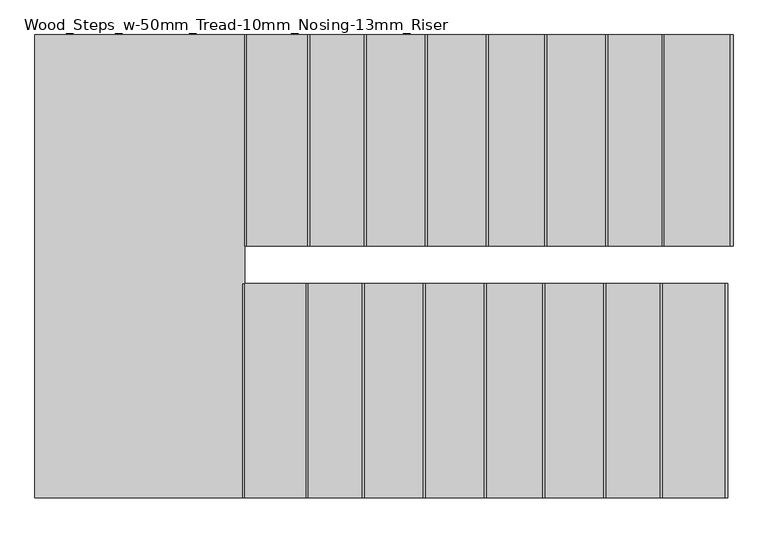
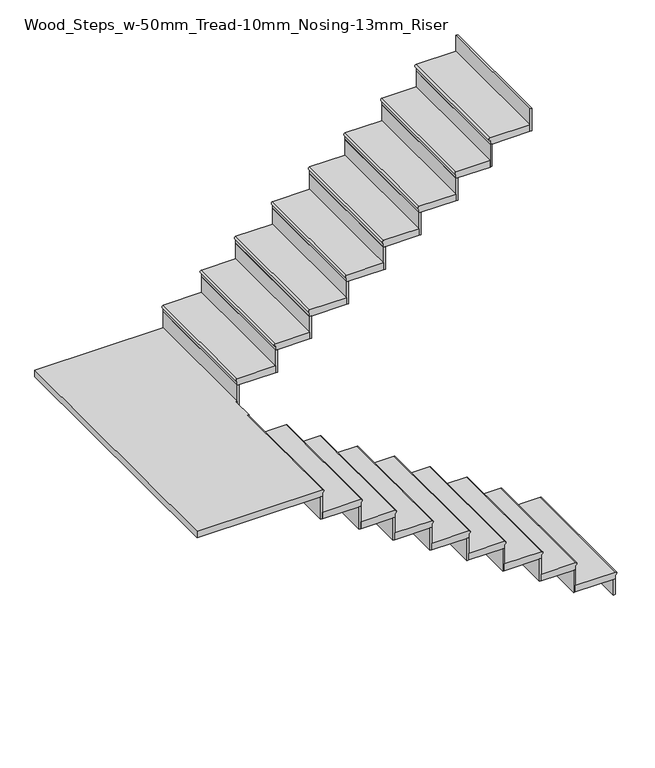
"""IFC4 building model written with IfcOpenShell, lengths in millimetres: stair flight geometry, Wood_Steps_w-50mm_Tread-10mm_Nosing-13mm_Riser."""

from ifc_helpers import new_model, si_unit, frame, origin, place, context, project, spatial, circle_curve, faceted_brep, source, transform, mapped, element, save
from ifc_brep_helpers import plane_surface, cylinder_surface, advanced_brep


def wood_steps_w_50mm_tread_10mm_nosing_13mm_riser_d55d0cb6(model_context):
    return source(origin(), model_context, "Body", "SolidModel", [
        advanced_brep(
        [(-5491.4951322, 1486.5182736, 146.6666667), (-5491.4951322, 1486.5182736, 166.6666667), (-5491.4951322, 572.7642586, 166.6666667), (-5491.4951322, 572.7642586, 146.6666667), (-5771.4951322, 572.7642586, 166.6666667), (-5771.4951322, 1486.5182736, 166.6666667), (-5491.4951322, 572.7642586, 116.6666667), (-5771.4951322, 572.7642586, 116.6666667), (-5771.4951322, 1486.5182736, 116.6666667), (-5491.4951322, 1486.5182736, 116.6666667)],
        [
            (0, 1, circle_curve(frame((-5491.4951322, 1486.5182736, 156.6666667), z_axis=(0.0, -1.0, 0.0), x_axis=(-1.0, 0.0, 0.0)), 10.0)),
            (1, 2),
            (2, 3, circle_curve(frame((-5491.4951322, 572.7642586, 156.6666667), z_axis=(0.0, 1.0, 0.0), x_axis=(-1.0, 0.0, 0.0)), 10.0)),
            (3, 0),
            (4, 2),
            (1, 5),
            (5, 4),
            (6, 7),
            (7, 8),
            (8, 9),
            (9, 6),
            (4, 7),
            (6, 3),
            (9, 0),
            (8, 5),
        ],
        [
            cylinder_surface(frame((-5491.4951322, 1486.5182736, 156.6666667), z_axis=(0.0, 1.0, 0.0), x_axis=(-1.0, 0.0, 0.0)), 10.0),
            plane_surface(frame((-5466.6718965, 572.7642586, 166.6666667), z_axis=(0.0, 0.0, 1.0), x_axis=(1.0, 0.0, 0.0))),
            plane_surface(frame((-5466.6718965, 572.7642586, 116.6666667), z_axis=(0.0, 0.0, -1.0), x_axis=(-1.0, 0.0, 0.0))),
            plane_surface(frame((-5771.4951322, 572.7642586, 166.6666667), z_axis=(0.0, -1.0, 0.0), x_axis=(0.0, 0.0, -1.0))),
            plane_surface(frame((-5491.4951322, 572.7642586, 166.6666667), z_axis=(1.0, 0.0, 0.0), x_axis=(0.0, 0.0, -1.0))),
            plane_surface(frame((-5491.4951322, 1486.5182736, 166.6666667), z_axis=(0.0, 1.0, 0.0), x_axis=(0.0, 0.0, -1.0))),
            plane_surface(frame((-5771.4951322, 1486.5182736, 166.6666667), z_axis=(-1.0, 0.0, 0.0), x_axis=(0.0, 0.0, -1.0))),
        ],
        [
            (0, [[1, 2, 3, 4]]),
            (1, [[5, -2, 6, 7]]),
            (2, [[8, 9, 10, 11]]),
            (3, [[-5, 12, -8, 13, -3]]),
            (4, [[-11, 14, -4, -13]]),
            (5, [[-6, -1, -14, -10, 15]]),
            (6, [[-7, -15, -9, -12]]),
        ],
    ),
        faceted_brep([(-5491.4951322, 1486.5182736, 116.6666667), (-5491.4951322, 1486.5182736, 0.0), (-5503.9951322, 1486.5182736, 0.0), (-5503.9951322, 1486.5182736, 116.6666667), (-5491.4951322, 572.7642586, 116.6666667), (-5503.9951322, 572.7642586, 116.6666667), (-5503.9951322, 572.7642586, 0.0), (-5491.4951322, 572.7642586, 0.0)], [[[0, 1, 2, 3]], [[4, 5, 6, 7]], [[1, 0, 4, 7]], [[2, 1, 7, 6]], [[3, 2, 6, 5]], [[0, 3, 5, 4]]]),
        faceted_brep([(-5771.4951322, 1486.5182736, 283.3333333), (-5771.4951322, 1486.5182736, 116.6666667), (-5783.9951322, 1486.5182736, 116.6666667), (-5783.9951322, 1486.5182736, 283.3333333), (-5771.4951322, 572.7642586, 283.3333333), (-5783.9951322, 572.7642586, 283.3333333), (-5783.9951322, 572.7642586, 116.6666667), (-5771.4951322, 572.7642586, 116.6666667)], [[[0, 1, 2, 3]], [[4, 5, 6, 7]], [[1, 0, 4, 7]], [[2, 1, 7, 6]], [[3, 2, 6, 5]], [[0, 3, 5, 4]]]),
        advanced_brep(
        [(-6011.4951322, 572.7642586, 333.3333333), (-5771.4951322, 572.7642586, 333.3333333), (-5771.4951322, 1486.5182736, 333.3333333), (-6011.4951322, 1486.5182736, 333.3333333), (-5771.4951322, 572.7642586, 283.3333333), (-6011.4951322, 572.7642586, 283.3333333), (-6011.4951322, 1486.5182736, 283.3333333), (-5771.4951322, 1486.5182736, 283.3333333), (-5771.4951322, 572.7642586, 313.3333333), (-5771.4951322, 1486.5182736, 313.3333333)],
        [
            (0, 1),
            (1, 2),
            (2, 3),
            (3, 0),
            (4, 5),
            (5, 6),
            (6, 7),
            (7, 4),
            (0, 5),
            (4, 8),
            (8, 1, circle_curve(frame((-5771.4951322, 572.7642586, 323.3333333), z_axis=(0.0, -1.0, 0.0), x_axis=(-1.0, 0.0, 0.0)), 10.0)),
            (7, 9),
            (9, 8),
            (2, 9, circle_curve(frame((-5771.4951322, 1486.5182736, 323.3333333), z_axis=(0.0, 1.0, 0.0), x_axis=(-1.0, 0.0, 0.0)), 10.0)),
            (6, 3),
        ],
        [
            plane_surface(frame((-5466.6718965, 572.7642586, 333.3333333), z_axis=(0.0, 0.0, 1.0), x_axis=(1.0, 0.0, 0.0))),
            plane_surface(frame((-5466.6718965, 572.7642586, 283.3333333), z_axis=(0.0, 0.0, -1.0), x_axis=(-1.0, 0.0, 0.0))),
            plane_surface(frame((-6011.4951322, 572.7642586, 333.3333333), z_axis=(0.0, -1.0, 0.0), x_axis=(0.0, 0.0, -1.0))),
            plane_surface(frame((-5771.4951322, 572.7642586, 333.3333333), z_axis=(1.0, 0.0, 0.0), x_axis=(0.0, 0.0, -1.0))),
            plane_surface(frame((-5771.4951322, 1486.5182736, 333.3333333), z_axis=(0.0, 1.0, 0.0), x_axis=(0.0, 0.0, -1.0))),
            plane_surface(frame((-6011.4951322, 1486.5182736, 333.3333333), z_axis=(-1.0, 0.0, 0.0), x_axis=(0.0, 0.0, -1.0))),
            cylinder_surface(frame((-5771.4951322, 1486.5182736, 323.3333333), z_axis=(0.0, 1.0, 0.0), x_axis=(-1.0, 0.0, 0.0)), 10.0),
        ],
        [
            (0, [[1, 2, 3, 4]]),
            (1, [[5, 6, 7, 8]]),
            (2, [[-1, 9, -5, 10, 11]]),
            (3, [[-8, 12, 13, -10]]),
            (4, [[-3, 14, -12, -7, 15]]),
            (5, [[-4, -15, -6, -9]]),
            (6, [[-14, -2, -11, -13]]),
        ],
    ),
        faceted_brep([(-6011.4951322, 1486.5182736, 450.0), (-6011.4951322, 1486.5182736, 283.3333333), (-6023.9951322, 1486.5182736, 283.3333333), (-6023.9951322, 1486.5182736, 450.0), (-6011.4951322, 572.7642586, 450.0), (-6023.9951322, 572.7642586, 450.0), (-6023.9951322, 572.7642586, 283.3333333), (-6011.4951322, 572.7642586, 283.3333333)], [[[0, 1, 2, 3]], [[4, 5, 6, 7]], [[1, 0, 4, 7]], [[2, 1, 7, 6]], [[3, 2, 6, 5]], [[0, 3, 5, 4]]]),
        advanced_brep(
        [(-6271.4951322, 572.7642586, 500.0), (-6011.4951322, 572.7642586, 500.0), (-6011.4951322, 1486.5182736, 500.0), (-6271.4951322, 1486.5182736, 500.0), (-6011.4951322, 572.7642586, 450.0), (-6271.4951322, 572.7642586, 450.0), (-6271.4951322, 1486.5182736, 450.0), (-6011.4951322, 1486.5182736, 450.0), (-6011.4951322, 572.7642586, 480.0), (-6011.4951322, 1486.5182736, 480.0)],
        [
            (0, 1),
            (1, 2),
            (2, 3),
            (3, 0),
            (4, 5),
            (5, 6),
            (6, 7),
            (7, 4),
            (0, 5),
            (4, 8),
            (8, 1, circle_curve(frame((-6011.4951322, 572.7642586, 490.0), z_axis=(0.0, -1.0, 0.0), x_axis=(-1.0, 0.0, 0.0)), 10.0)),
            (7, 9),
            (9, 8),
            (2, 9, circle_curve(frame((-6011.4951322, 1486.5182736, 490.0), z_axis=(0.0, 1.0, 0.0), x_axis=(-1.0, 0.0, 0.0)), 10.0)),
            (6, 3),
        ],
        [
            plane_surface(frame((-5466.6718965, 572.7642586, 500.0), z_axis=(0.0, 0.0, 1.0), x_axis=(1.0, 0.0, 0.0))),
            plane_surface(frame((-5466.6718965, 572.7642586, 450.0), z_axis=(0.0, 0.0, -1.0), x_axis=(-1.0, 0.0, 0.0))),
            plane_surface(frame((-6271.4951322, 572.7642586, 500.0), z_axis=(0.0, -1.0, 0.0), x_axis=(0.0, 0.0, -1.0))),
            plane_surface(frame((-6011.4951322, 572.7642586, 500.0), z_axis=(1.0, 0.0, 0.0), x_axis=(0.0, 0.0, -1.0))),
            plane_surface(frame((-6011.4951322, 1486.5182736, 500.0), z_axis=(0.0, 1.0, 0.0), x_axis=(0.0, 0.0, -1.0))),
            plane_surface(frame((-6271.4951322, 1486.5182736, 500.0), z_axis=(-1.0, 0.0, 0.0), x_axis=(0.0, 0.0, -1.0))),
            cylinder_surface(frame((-6011.4951322, 1486.5182736, 490.0), z_axis=(0.0, 1.0, 0.0), x_axis=(-1.0, 0.0, 0.0)), 10.0),
        ],
        [
            (0, [[1, 2, 3, 4]]),
            (1, [[5, 6, 7, 8]]),
            (2, [[-1, 9, -5, 10, 11]]),
            (3, [[-8, 12, 13, -10]]),
            (4, [[-3, 14, -12, -7, 15]]),
            (5, [[-4, -15, -6, -9]]),
            (6, [[-14, -2, -11, -13]]),
        ],
    ),
        faceted_brep([(-6271.4951322, 1486.5182736, 616.6666667), (-6271.4951322, 1486.5182736, 450.0), (-6283.9951322, 1486.5182736, 450.0), (-6283.9951322, 1486.5182736, 616.6666667), (-6271.4951322, 572.7642586, 616.6666667), (-6283.9951322, 572.7642586, 616.6666667), (-6283.9951322, 572.7642586, 450.0), (-6271.4951322, 572.7642586, 450.0)], [[[0, 1, 2, 3]], [[4, 5, 6, 7]], [[1, 0, 4, 7]], [[2, 1, 7, 6]], [[3, 2, 6, 5]], [[0, 3, 5, 4]]]),
        advanced_brep(
        [(-6521.4951322, 572.7642586, 666.6666667), (-6271.4951322, 572.7642586, 666.6666667), (-6271.4951322, 1486.5182736, 666.6666667), (-6521.4951322, 1486.5182736, 666.6666667), (-6271.4951322, 572.7642586, 616.6666667), (-6521.4951322, 572.7642586, 616.6666667), (-6521.4951322, 1486.5182736, 616.6666667), (-6271.4951322, 1486.5182736, 616.6666667), (-6271.4951322, 572.7642586, 646.6666667), (-6271.4951322, 1486.5182736, 646.6666667)],
        [
            (0, 1),
            (1, 2),
            (2, 3),
            (3, 0),
            (4, 5),
            (5, 6),
            (6, 7),
            (7, 4),
            (0, 5),
            (4, 8),
            (8, 1, circle_curve(frame((-6271.4951322, 572.7642586, 656.6666667), z_axis=(0.0, -1.0, 0.0), x_axis=(-1.0, 0.0, 0.0)), 10.0)),
            (7, 9),
            (9, 8),
            (2, 9, circle_curve(frame((-6271.4951322, 1486.5182736, 656.6666667), z_axis=(0.0, 1.0, 0.0), x_axis=(-1.0, 0.0, 0.0)), 10.0)),
            (6, 3),
        ],
        [
            plane_surface(frame((-5466.6718965, 572.7642586, 666.6666667), z_axis=(0.0, 0.0, 1.0), x_axis=(1.0, 0.0, 0.0))),
            plane_surface(frame((-5466.6718965, 572.7642586, 616.6666667), z_axis=(0.0, 0.0, -1.0), x_axis=(-1.0, 0.0, 0.0))),
            plane_surface(frame((-6521.4951322, 572.7642586, 666.6666667), z_axis=(0.0, -1.0, 0.0), x_axis=(0.0, 0.0, -1.0))),
            plane_surface(frame((-6271.4951322, 572.7642586, 666.6666667), z_axis=(1.0, 0.0, 0.0), x_axis=(0.0, 0.0, -1.0))),
            plane_surface(frame((-6271.4951322, 1486.5182736, 666.6666667), z_axis=(0.0, 1.0, 0.0), x_axis=(0.0, 0.0, -1.0))),
            plane_surface(frame((-6521.4951322, 1486.5182736, 666.6666667), z_axis=(-1.0, 0.0, 0.0), x_axis=(0.0, 0.0, -1.0))),
            cylinder_surface(frame((-6271.4951322, 1486.5182736, 656.6666667), z_axis=(0.0, 1.0, 0.0), x_axis=(-1.0, 0.0, 0.0)), 10.0),
        ],
        [
            (0, [[1, 2, 3, 4]]),
            (1, [[5, 6, 7, 8]]),
            (2, [[-1, 9, -5, 10, 11]]),
            (3, [[-8, 12, 13, -10]]),
            (4, [[-3, 14, -12, -7, 15]]),
            (5, [[-4, -15, -6, -9]]),
            (6, [[-14, -2, -11, -13]]),
        ],
    ),
        faceted_brep([(-6521.4951322, 1486.5182736, 783.3333333), (-6521.4951322, 1486.5182736, 616.6666667), (-6533.9951322, 1486.5182736, 616.6666667), (-6533.9951322, 1486.5182736, 783.3333333), (-6521.4951322, 572.7642586, 783.3333333), (-6533.9951322, 572.7642586, 783.3333333), (-6533.9951322, 572.7642586, 616.6666667), (-6521.4951322, 572.7642586, 616.6666667)], [[[0, 1, 2, 3]], [[4, 5, 6, 7]], [[1, 0, 4, 7]], [[2, 1, 7, 6]], [[3, 2, 6, 5]], [[0, 3, 5, 4]]]),
        advanced_brep(
        [(-6781.4951322, 572.7642586, 833.3333333), (-6521.4951322, 572.7642586, 833.3333333), (-6521.4951322, 1486.5182736, 833.3333333), (-6781.4951322, 1486.5182736, 833.3333333), (-6521.4951322, 572.7642586, 783.3333333), (-6781.4951322, 572.7642586, 783.3333333), (-6781.4951322, 1486.5182736, 783.3333333), (-6521.4951322, 1486.5182736, 783.3333333), (-6521.4951322, 572.7642586, 813.3333333), (-6521.4951322, 1486.5182736, 813.3333333)],
        [
            (0, 1),
            (1, 2),
            (2, 3),
            (3, 0),
            (4, 5),
            (5, 6),
            (6, 7),
            (7, 4),
            (0, 5),
            (4, 8),
            (8, 1, circle_curve(frame((-6521.4951322, 572.7642586, 823.3333333), z_axis=(0.0, -1.0, 0.0), x_axis=(-1.0, 0.0, 0.0)), 10.0)),
            (7, 9),
            (9, 8),
            (2, 9, circle_curve(frame((-6521.4951322, 1486.5182736, 823.3333333), z_axis=(0.0, 1.0, 0.0), x_axis=(-1.0, 0.0, 0.0)), 10.0)),
            (6, 3),
        ],
        [
            plane_surface(frame((-5466.6718965, 572.7642586, 833.3333333), z_axis=(0.0, 0.0, 1.0), x_axis=(1.0, 0.0, 0.0))),
            plane_surface(frame((-5466.6718965, 572.7642586, 783.3333333), z_axis=(0.0, 0.0, -1.0), x_axis=(-1.0, 0.0, 0.0))),
            plane_surface(frame((-6781.4951322, 572.7642586, 833.3333333), z_axis=(0.0, -1.0, 0.0), x_axis=(0.0, 0.0, -1.0))),
            plane_surface(frame((-6521.4951322, 572.7642586, 833.3333333), z_axis=(1.0, 0.0, 0.0), x_axis=(0.0, 0.0, -1.0))),
            plane_surface(frame((-6521.4951322, 1486.5182736, 833.3333333), z_axis=(0.0, 1.0, 0.0), x_axis=(0.0, 0.0, -1.0))),
            plane_surface(frame((-6781.4951322, 1486.5182736, 833.3333333), z_axis=(-1.0, 0.0, 0.0), x_axis=(0.0, 0.0, -1.0))),
            cylinder_surface(frame((-6521.4951322, 1486.5182736, 823.3333333), z_axis=(0.0, 1.0, 0.0), x_axis=(-1.0, 0.0, 0.0)), 10.0),
        ],
        [
            (0, [[1, 2, 3, 4]]),
            (1, [[5, 6, 7, 8]]),
            (2, [[-1, 9, -5, 10, 11]]),
            (3, [[-8, 12, 13, -10]]),
            (4, [[-3, 14, -12, -7, 15]]),
            (5, [[-4, -15, -6, -9]]),
            (6, [[-14, -2, -11, -13]]),
        ],
    ),
        faceted_brep([(-6781.4951322, 1486.5182736, 950.0), (-6781.4951322, 1486.5182736, 783.3333333), (-6793.9951322, 1486.5182736, 783.3333333), (-6793.9951322, 1486.5182736, 950.0), (-6781.4951322, 572.7642586, 950.0), (-6793.9951322, 572.7642586, 950.0), (-6793.9951322, 572.7642586, 783.3333333), (-6781.4951322, 572.7642586, 783.3333333)], [[[0, 1, 2, 3]], [[4, 5, 6, 7]], [[1, 0, 4, 7]], [[2, 1, 7, 6]], [[3, 2, 6, 5]], [[0, 3, 5, 4]]]),
        advanced_brep(
        [(-7041.4951322, 572.7642586, 1000.0), (-6781.4951322, 572.7642586, 1000.0), (-6781.4951322, 1486.5182736, 1000.0), (-7041.4951322, 1486.5182736, 1000.0), (-6781.4951322, 572.7642586, 950.0), (-7041.4951322, 572.7642586, 950.0), (-7041.4951322, 1486.5182736, 950.0), (-6781.4951322, 1486.5182736, 950.0), (-6781.4951322, 572.7642586, 980.0), (-6781.4951322, 1486.5182736, 980.0)],
        [
            (0, 1),
            (1, 2),
            (2, 3),
            (3, 0),
            (4, 5),
            (5, 6),
            (6, 7),
            (7, 4),
            (0, 5),
            (4, 8),
            (8, 1, circle_curve(frame((-6781.4951322, 572.7642586, 990.0), z_axis=(0.0, -1.0, 0.0), x_axis=(-1.0, 0.0, 0.0)), 10.0)),
            (7, 9),
            (9, 8),
            (2, 9, circle_curve(frame((-6781.4951322, 1486.5182736, 990.0), z_axis=(0.0, 1.0, 0.0), x_axis=(-1.0, 0.0, 0.0)), 10.0)),
            (6, 3),
        ],
        [
            plane_surface(frame((-5726.6718965, 572.7642586, 1000.0), z_axis=(0.0, 0.0, 1.0), x_axis=(1.0, 0.0, 0.0))),
            plane_surface(frame((-5726.6718965, 572.7642586, 950.0), z_axis=(0.0, 0.0, -1.0), x_axis=(-1.0, 0.0, 0.0))),
            plane_surface(frame((-7041.4951322, 572.7642586, 1000.0), z_axis=(0.0, -1.0, 0.0), x_axis=(0.0, 0.0, -1.0))),
            plane_surface(frame((-6781.4951322, 572.7642586, 1000.0), z_axis=(1.0, 0.0, 0.0), x_axis=(0.0, 0.0, -1.0))),
            plane_surface(frame((-6781.4951322, 1486.5182736, 1000.0), z_axis=(0.0, 1.0, 0.0), x_axis=(0.0, 0.0, -1.0))),
            plane_surface(frame((-7041.4951322, 1486.5182736, 1000.0), z_axis=(-1.0, 0.0, 0.0), x_axis=(0.0, 0.0, -1.0))),
            cylinder_surface(frame((-6781.4951322, 1486.5182736, 990.0), z_axis=(0.0, 1.0, 0.0), x_axis=(-1.0, 0.0, 0.0)), 10.0),
        ],
        [
            (0, [[1, 2, 3, 4]]),
            (1, [[5, 6, 7, 8]]),
            (2, [[-1, 9, -5, 10, 11]]),
            (3, [[-8, 12, 13, -10]]),
            (4, [[-3, 14, -12, -7, 15]]),
            (5, [[-4, -15, -6, -9]]),
            (6, [[-14, -2, -11, -13]]),
        ],
    ),
        faceted_brep([(-7041.4951322, 1486.5182736, 1116.6666667), (-7041.4951322, 1486.5182736, 950.0), (-7053.9951322, 1486.5182736, 950.0), (-7053.9951322, 1486.5182736, 1116.6666667), (-7041.4951322, 572.7642586, 1116.6666667), (-7053.9951322, 572.7642586, 1116.6666667), (-7053.9951322, 572.7642586, 950.0), (-7041.4951322, 572.7642586, 950.0)], [[[0, 1, 2, 3]], [[4, 5, 6, 7]], [[1, 0, 4, 7]], [[2, 1, 7, 6]], [[3, 2, 6, 5]], [[0, 3, 5, 4]]]),
        advanced_brep(
        [(-7281.4951322, 572.7642586, 1166.6666667), (-7041.4951322, 572.7642586, 1166.6666667), (-7041.4951322, 1486.5182736, 1166.6666667), (-7281.4951322, 1486.5182736, 1166.6666667), (-7041.4951322, 572.7642586, 1116.6666667), (-7281.4951322, 572.7642586, 1116.6666667), (-7281.4951322, 1486.5182736, 1116.6666667), (-7041.4951322, 1486.5182736, 1116.6666667), (-7041.4951322, 572.7642586, 1146.6666667), (-7041.4951322, 1486.5182736, 1146.6666667)],
        [
            (0, 1),
            (1, 2),
            (2, 3),
            (3, 0),
            (4, 5),
            (5, 6),
            (6, 7),
            (7, 4),
            (0, 5),
            (4, 8),
            (8, 1, circle_curve(frame((-7041.4951322, 572.7642586, 1156.6666667), z_axis=(0.0, -1.0, 0.0), x_axis=(-1.0, 0.0, 0.0)), 10.0)),
            (7, 9),
            (9, 8),
            (2, 9, circle_curve(frame((-7041.4951322, 1486.5182736, 1156.6666667), z_axis=(0.0, 1.0, 0.0), x_axis=(-1.0, 0.0, 0.0)), 10.0)),
            (6, 3),
        ],
        [
            plane_surface(frame((-5466.6718965, 572.7642586, 1166.6666667), z_axis=(0.0, 0.0, 1.0), x_axis=(1.0, 0.0, 0.0))),
            plane_surface(frame((-5466.6718965, 572.7642586, 1116.6666667), z_axis=(0.0, 0.0, -1.0), x_axis=(-1.0, 0.0, 0.0))),
            plane_surface(frame((-7281.4951322, 572.7642586, 1166.6666667), z_axis=(0.0, -1.0, 0.0), x_axis=(0.0, 0.0, -1.0))),
            plane_surface(frame((-7041.4951322, 572.7642586, 1166.6666667), z_axis=(1.0, 0.0, 0.0), x_axis=(0.0, 0.0, -1.0))),
            plane_surface(frame((-7041.4951322, 1486.5182736, 1166.6666667), z_axis=(0.0, 1.0, 0.0), x_axis=(0.0, 0.0, -1.0))),
            plane_surface(frame((-7281.4951322, 1486.5182736, 1166.6666667), z_axis=(-1.0, 0.0, 0.0), x_axis=(0.0, 0.0, -1.0))),
            cylinder_surface(frame((-7041.4951322, 1486.5182736, 1156.6666667), z_axis=(0.0, 1.0, 0.0), x_axis=(-1.0, 0.0, 0.0)), 10.0),
        ],
        [
            (0, [[1, 2, 3, 4]]),
            (1, [[5, 6, 7, 8]]),
            (2, [[-1, 9, -5, 10, 11]]),
            (3, [[-8, 12, 13, -10]]),
            (4, [[-3, 14, -12, -7, 15]]),
            (5, [[-4, -15, -6, -9]]),
            (6, [[-14, -2, -11, -13]]),
        ],
    ),
        faceted_brep([(-7281.4951322, 1486.5182736, 1283.3333333), (-7281.4951322, 1486.5182736, 1116.6666667), (-7293.9951322, 1486.5182736, 1116.6666667), (-7293.9951322, 1486.5182736, 1283.3333333), (-7281.4951322, 572.7642586, 1283.3333333), (-7293.9951322, 572.7642586, 1283.3333333), (-7293.9951322, 572.7642586, 1116.6666667), (-7281.4951322, 572.7642586, 1116.6666667)], [[[0, 1, 2, 3]], [[4, 5, 6, 7]], [[1, 0, 4, 7]], [[2, 1, 7, 6]], [[3, 2, 6, 5]], [[0, 3, 5, 4]]]),
        advanced_brep(
        [(-7551.4951322, 572.7642586, 1333.3333333), (-7281.4951322, 572.7642586, 1333.3333333), (-7281.4951322, 1486.5182736, 1333.3333333), (-7551.4951322, 1486.5182736, 1333.3333333), (-7281.4951322, 572.7642586, 1283.3333333), (-7551.4951322, 572.7642586, 1283.3333333), (-7551.4951322, 1486.5182736, 1283.3333333), (-7281.4951322, 1486.5182736, 1283.3333333), (-7281.4951322, 572.7642586, 1313.3333333), (-7281.4951322, 1486.5182736, 1313.3333333)],
        [
            (0, 1),
            (1, 2),
            (2, 3),
            (3, 0),
            (4, 5),
            (5, 6),
            (6, 7),
            (7, 4),
            (0, 5),
            (4, 8),
            (8, 1, circle_curve(frame((-7281.4951322, 572.7642586, 1323.3333333), z_axis=(0.0, -1.0, 0.0), x_axis=(-1.0, 0.0, 0.0)), 10.0)),
            (7, 9),
            (9, 8),
            (2, 9, circle_curve(frame((-7281.4951322, 1486.5182736, 1323.3333333), z_axis=(0.0, 1.0, 0.0), x_axis=(-1.0, 0.0, 0.0)), 10.0)),
            (6, 3),
        ],
        [
            plane_surface(frame((-5466.6718965, 572.7642586, 1333.3333333), z_axis=(0.0, 0.0, 1.0), x_axis=(1.0, 0.0, 0.0))),
            plane_surface(frame((-5466.6718965, 572.7642586, 1283.3333333), z_axis=(0.0, 0.0, -1.0), x_axis=(-1.0, 0.0, 0.0))),
            plane_surface(frame((-7551.4951322, 572.7642586, 1333.3333333), z_axis=(0.0, -1.0, 0.0), x_axis=(0.0, 0.0, -1.0))),
            plane_surface(frame((-7281.4951322, 572.7642586, 1333.3333333), z_axis=(1.0, 0.0, 0.0), x_axis=(0.0, 0.0, -1.0))),
            plane_surface(frame((-7281.4951322, 1486.5182736, 1333.3333333), z_axis=(0.0, 1.0, 0.0), x_axis=(0.0, 0.0, -1.0))),
            plane_surface(frame((-7551.4951322, 1486.5182736, 1333.3333333), z_axis=(-1.0, 0.0, 0.0), x_axis=(0.0, 0.0, -1.0))),
            cylinder_surface(frame((-7281.4951322, 1486.5182736, 1323.3333333), z_axis=(0.0, 1.0, 0.0), x_axis=(-1.0, 0.0, 0.0)), 10.0),
        ],
        [
            (0, [[1, 2, 3, 4]]),
            (1, [[5, 6, 7, 8]]),
            (2, [[-1, 9, -5, 10, 11]]),
            (3, [[-8, 12, 13, -10]]),
            (4, [[-3, 14, -12, -7, 15]]),
            (5, [[-4, -15, -6, -9]]),
            (6, [[-14, -2, -11, -13]]),
        ],
    ),
        faceted_brep([(-7551.4951322, 1486.5182736, 1450.0), (-7551.4951322, 1486.5182736, 1283.3333333), (-7563.9951322, 1486.5182736, 1283.3333333), (-7563.9951322, 1486.5182736, 1450.0), (-7551.4951322, 572.7642586, 1450.0), (-7563.9951322, 572.7642586, 1450.0), (-7563.9951322, 572.7642586, 1283.3333333), (-7551.4951322, 572.7642586, 1283.3333333)], [[[0, 1, 2, 3]], [[4, 5, 6, 7]], [[1, 0, 4, 7]], [[2, 1, 7, 6]], [[3, 2, 6, 5]], [[0, 3, 5, 4]]]),
        advanced_brep(
        [(-7531.4951322, 2546.998858, 1500.0), (-8434.8904087, 2546.998858, 1500.0), (-8434.8904087, 572.7642586, 1500.0), (-7551.4951322, 572.7642586, 1500.0), (-7551.4951322, 1486.5182736, 1500.0), (-7541.4951322, 1486.5182736, 1500.0), (-7541.4951322, 1646.5182736, 1500.0), (-7531.4951322, 1646.5182736, 1500.0), (-8434.8904087, 2546.998858, 1450.0), (-7531.4951322, 2546.998858, 1450.0), (-7531.4951322, 1646.5182736, 1450.0), (-7541.4951322, 1646.5182736, 1450.0), (-7541.4951322, 1486.5182736, 1450.0), (-7551.4951322, 1486.5182736, 1450.0), (-7551.4951322, 572.7642586, 1450.0), (-8434.8904087, 572.7642586, 1450.0), (-7551.4951322, 572.7642586, 1480.0), (-7551.4951322, 1486.5182736, 1480.0), (-7541.4951322, 1486.5182736, 1490.0)],
        [
            (0, 1),
            (1, 2),
            (2, 3),
            (3, 4),
            (4, 5),
            (5, 6),
            (6, 7),
            (7, 0),
            (8, 9),
            (9, 10),
            (10, 11),
            (11, 12),
            (12, 13),
            (13, 14),
            (14, 15),
            (15, 8),
            (0, 9),
            (8, 1),
            (15, 2),
            (14, 16),
            (16, 3, circle_curve(frame((-7551.4951322, 572.7642586, 1490.0), z_axis=(0.0, -1.0, 0.0), x_axis=(-1.0, 0.0, 0.0)), 10.0)),
            (13, 17),
            (17, 16),
            (4, 18, circle_curve(frame((-7551.4951322, 1486.5182736, 1490.0), z_axis=(0.0, 1.0, 0.0), x_axis=(-1.0, 0.0, 0.0)), 10.0)),
            (18, 5),
            (12, 18),
            (18, 17, circle_curve(frame((-7551.4951322, 1486.5182736, 1490.0), z_axis=(0.0, 1.0, 0.0), x_axis=(-1.0, 0.0, 0.0)), 10.0)),
            (11, 6),
            (10, 7),
        ],
        [
            plane_surface(frame((-8434.8904087, 2546.998858, 1500.0), z_axis=(0.0, 0.0, 1.0), x_axis=(-1.0, 0.0, 0.0))),
            plane_surface(frame((-8434.8904087, 2546.998858, 1450.0), z_axis=(0.0, 0.0, -1.0), x_axis=(1.0, 0.0, 0.0))),
            plane_surface(frame((-7531.4951322, 2546.998858, 1500.0), z_axis=(0.0, 1.0, 0.0), x_axis=(0.0, 0.0, -1.0))),
            plane_surface(frame((-8434.8904087, 2546.998858, 1500.0), z_axis=(-1.0, 0.0, 0.0), x_axis=(0.0, 0.0, -1.0))),
            plane_surface(frame((-8434.8904087, 572.7642586, 1500.0), z_axis=(0.0, -1.0, 0.0), x_axis=(0.0, 0.0, -1.0))),
            plane_surface(frame((-7551.4951322, 572.7642586, 1500.0), z_axis=(1.0, 0.0, 0.0), x_axis=(0.0, 0.0, -1.0))),
            plane_surface(frame((-7551.4951322, 1486.5182736, 1500.0), z_axis=(0.0, -1.0, 0.0), x_axis=(0.0, 0.0, -1.0))),
            plane_surface(frame((-7541.4951322, 1486.5182736, 1500.0), z_axis=(1.0, 0.0, 0.0), x_axis=(0.0, 0.0, -1.0))),
            plane_surface(frame((-7541.4951322, 1646.5182736, 1500.0), z_axis=(0.0, -1.0, 0.0), x_axis=(0.0, 0.0, -1.0))),
            plane_surface(frame((-7531.4951322, 1646.5182736, 1500.0), z_axis=(1.0, 0.0, 0.0), x_axis=(0.0, 0.0, -1.0))),
            cylinder_surface(frame((-7551.4951322, 1486.5182736, 1490.0), z_axis=(0.0, 1.0, 0.0), x_axis=(-1.0, 0.0, 0.0)), 10.0),
        ],
        [
            (0, [[1, 2, 3, 4, 5, 6, 7, 8]]),
            (1, [[9, 10, 11, 12, 13, 14, 15, 16]]),
            (2, [[-1, 17, -9, 18]]),
            (3, [[-2, -18, -16, 19]]),
            (4, [[-3, -19, -15, 20, 21]]),
            (5, [[-14, 22, 23, -20]]),
            (6, [[-5, 24, 25]]),
            (6, [[-13, 26, 27, -22]]),
            (7, [[-6, -25, -26, -12, 28]]),
            (8, [[-7, -28, -11, 29]]),
            (9, [[-8, -29, -10, -17]]),
            (10, [[-21, -23, -27, -24, -4]]),
        ],
    ),
        faceted_brep([(-7531.4951322, 1646.5182736, 1616.6666667), (-7531.4951322, 1646.5182736, 1450.0), (-7518.9951322, 1646.5182736, 1450.0), (-7518.9951322, 1646.5182736, 1616.6666667), (-7531.4951322, 2546.998858, 1616.6666667), (-7518.9951322, 2546.998858, 1616.6666667), (-7518.9951322, 2546.998858, 1450.0), (-7531.4951322, 2546.998858, 1450.0)], [[[0, 1, 2, 3]], [[4, 5, 6, 7]], [[1, 0, 4, 7]], [[2, 1, 7, 6]], [[3, 2, 6, 5]], [[0, 3, 5, 4]]]),
        advanced_brep(
        [(-7261.4951322, 2546.998858, 1666.6666667), (-7531.4951322, 2546.998858, 1666.6666667), (-7531.4951322, 1646.5182736, 1666.6666667), (-7261.4951322, 1646.5182736, 1666.6666667), (-7531.4951322, 2546.998858, 1616.6666667), (-7261.4951322, 2546.998858, 1616.6666667), (-7261.4951322, 1646.5182736, 1616.6666667), (-7531.4951322, 1646.5182736, 1616.6666667), (-7531.4951322, 2546.998858, 1646.6666667), (-7531.4951322, 1646.5182736, 1646.6666667)],
        [
            (0, 1),
            (1, 2),
            (2, 3),
            (3, 0),
            (4, 5),
            (5, 6),
            (6, 7),
            (7, 4),
            (0, 5),
            (4, 8),
            (8, 1, circle_curve(frame((-7531.4951322, 2546.998858, 1656.6666667), z_axis=(0.0, 1.0, 0.0), x_axis=(1.0, 0.0, 0.0)), 10.0)),
            (7, 9),
            (9, 8),
            (2, 9, circle_curve(frame((-7531.4951322, 1646.5182736, 1656.6666667), z_axis=(0.0, -1.0, 0.0), x_axis=(1.0, 0.0, 0.0)), 10.0)),
            (6, 3),
        ],
        [
            plane_surface(frame((-8434.8904087, 2546.998858, 1666.6666667), z_axis=(0.0, 0.0, 1.0), x_axis=(-1.0, 0.0, 0.0))),
            plane_surface(frame((-8434.8904087, 2546.998858, 1616.6666667), z_axis=(0.0, 0.0, -1.0), x_axis=(1.0, 0.0, 0.0))),
            plane_surface(frame((-7261.4951322, 2546.998858, 1666.6666667), z_axis=(0.0, 1.0, 0.0), x_axis=(0.0, 0.0, -1.0))),
            plane_surface(frame((-7531.4951322, 2546.998858, 1666.6666667), z_axis=(-1.0, 0.0, 0.0), x_axis=(0.0, 0.0, -1.0))),
            plane_surface(frame((-7531.4951322, 1646.5182736, 1666.6666667), z_axis=(0.0, -1.0, 0.0), x_axis=(0.0, 0.0, -1.0))),
            plane_surface(frame((-7261.4951322, 1646.5182736, 1666.6666667), z_axis=(1.0, 0.0, 0.0), x_axis=(0.0, 0.0, -1.0))),
            cylinder_surface(frame((-7531.4951322, 1646.5182736, 1656.6666667), z_axis=(0.0, -1.0, 0.0), x_axis=(1.0, 0.0, 0.0)), 10.0),
        ],
        [
            (0, [[1, 2, 3, 4]]),
            (1, [[5, 6, 7, 8]]),
            (2, [[-1, 9, -5, 10, 11]]),
            (3, [[-8, 12, 13, -10]]),
            (4, [[-3, 14, -12, -7, 15]]),
            (5, [[-4, -15, -6, -9]]),
            (6, [[-14, -2, -11, -13]]),
        ],
    ),
        faceted_brep([(-7261.4951322, 1646.5182736, 1783.3333333), (-7261.4951322, 1646.5182736, 1616.6666667), (-7248.9951322, 1646.5182736, 1616.6666667), (-7248.9951322, 1646.5182736, 1783.3333333), (-7261.4951322, 2546.998858, 1783.3333333), (-7248.9951322, 2546.998858, 1783.3333333), (-7248.9951322, 2546.998858, 1616.6666667), (-7261.4951322, 2546.998858, 1616.6666667)], [[[0, 1, 2, 3]], [[4, 5, 6, 7]], [[1, 0, 4, 7]], [[2, 1, 7, 6]], [[3, 2, 6, 5]], [[0, 3, 5, 4]]]),
        advanced_brep(
        [(-7021.4951322, 2546.998858, 1833.3333333), (-7261.4951322, 2546.998858, 1833.3333333), (-7261.4951322, 1646.5182736, 1833.3333333), (-7021.4951322, 1646.5182736, 1833.3333333), (-7261.4951322, 2546.998858, 1783.3333333), (-7021.4951322, 2546.998858, 1783.3333333), (-7021.4951322, 1646.5182736, 1783.3333333), (-7261.4951322, 1646.5182736, 1783.3333333), (-7261.4951322, 2546.998858, 1813.3333333), (-7261.4951322, 1646.5182736, 1813.3333333)],
        [
            (0, 1),
            (1, 2),
            (2, 3),
            (3, 0),
            (4, 5),
            (5, 6),
            (6, 7),
            (7, 4),
            (0, 5),
            (4, 8),
            (8, 1, circle_curve(frame((-7261.4951322, 2546.998858, 1823.3333333), z_axis=(0.0, 1.0, 0.0), x_axis=(1.0, 0.0, 0.0)), 10.0)),
            (7, 9),
            (9, 8),
            (2, 9, circle_curve(frame((-7261.4951322, 1646.5182736, 1823.3333333), z_axis=(0.0, -1.0, 0.0), x_axis=(1.0, 0.0, 0.0)), 10.0)),
            (6, 3),
        ],
        [
            plane_surface(frame((-8434.8904087, 2546.998858, 1833.3333333), z_axis=(0.0, 0.0, 1.0), x_axis=(-1.0, 0.0, 0.0))),
            plane_surface(frame((-8434.8904087, 2546.998858, 1783.3333333), z_axis=(0.0, 0.0, -1.0), x_axis=(1.0, 0.0, 0.0))),
            plane_surface(frame((-7021.4951322, 2546.998858, 1833.3333333), z_axis=(0.0, 1.0, 0.0), x_axis=(0.0, 0.0, -1.0))),
            plane_surface(frame((-7261.4951322, 2546.998858, 1833.3333333), z_axis=(-1.0, 0.0, 0.0), x_axis=(0.0, 0.0, -1.0))),
            plane_surface(frame((-7261.4951322, 1646.5182736, 1833.3333333), z_axis=(0.0, -1.0, 0.0), x_axis=(0.0, 0.0, -1.0))),
            plane_surface(frame((-7021.4951322, 1646.5182736, 1833.3333333), z_axis=(1.0, 0.0, 0.0), x_axis=(0.0, 0.0, -1.0))),
            cylinder_surface(frame((-7261.4951322, 1646.5182736, 1823.3333333), z_axis=(0.0, -1.0, 0.0), x_axis=(1.0, 0.0, 0.0)), 10.0),
        ],
        [
            (0, [[1, 2, 3, 4]]),
            (1, [[5, 6, 7, 8]]),
            (2, [[-1, 9, -5, 10, 11]]),
            (3, [[-8, 12, 13, -10]]),
            (4, [[-3, 14, -12, -7, 15]]),
            (5, [[-4, -15, -6, -9]]),
            (6, [[-14, -2, -11, -13]]),
        ],
    ),
        faceted_brep([(-7021.4951322, 1646.5182736, 1950.0), (-7021.4951322, 1646.5182736, 1783.3333333), (-7008.9951322, 1646.5182736, 1783.3333333), (-7008.9951322, 1646.5182736, 1950.0), (-7021.4951322, 2546.998858, 1950.0), (-7008.9951322, 2546.998858, 1950.0), (-7008.9951322, 2546.998858, 1783.3333333), (-7021.4951322, 2546.998858, 1783.3333333)], [[[0, 1, 2, 3]], [[4, 5, 6, 7]], [[1, 0, 4, 7]], [[2, 1, 7, 6]], [[3, 2, 6, 5]], [[0, 3, 5, 4]]]),
        advanced_brep(
        [(-6761.4951322, 2546.998858, 2000.0), (-7021.4951322, 2546.998858, 2000.0), (-7021.4951322, 1646.5182736, 2000.0), (-6761.4951322, 1646.5182736, 2000.0), (-7021.4951322, 2546.998858, 1950.0), (-6761.4951322, 2546.998858, 1950.0), (-6761.4951322, 1646.5182736, 1950.0), (-7021.4951322, 1646.5182736, 1950.0), (-7021.4951322, 2546.998858, 1980.0), (-7021.4951322, 1646.5182736, 1980.0)],
        [
            (0, 1),
            (1, 2),
            (2, 3),
            (3, 0),
            (4, 5),
            (5, 6),
            (6, 7),
            (7, 4),
            (0, 5),
            (4, 8),
            (8, 1, circle_curve(frame((-7021.4951322, 2546.998858, 1990.0), z_axis=(0.0, 1.0, 0.0), x_axis=(1.0, 0.0, 0.0)), 10.0)),
            (7, 9),
            (9, 8),
            (2, 9, circle_curve(frame((-7021.4951322, 1646.5182736, 1990.0), z_axis=(0.0, -1.0, 0.0), x_axis=(1.0, 0.0, 0.0)), 10.0)),
            (6, 3),
        ],
        [
            plane_surface(frame((-8434.8904087, 2546.998858, 2000.0), z_axis=(0.0, 0.0, 1.0), x_axis=(-1.0, 0.0, 0.0))),
            plane_surface(frame((-8434.8904087, 2546.998858, 1950.0), z_axis=(0.0, 0.0, -1.0), x_axis=(1.0, 0.0, 0.0))),
            plane_surface(frame((-6761.4951322, 2546.998858, 2000.0), z_axis=(0.0, 1.0, 0.0), x_axis=(0.0, 0.0, -1.0))),
            plane_surface(frame((-7021.4951322, 2546.998858, 2000.0), z_axis=(-1.0, 0.0, 0.0), x_axis=(0.0, 0.0, -1.0))),
            plane_surface(frame((-7021.4951322, 1646.5182736, 2000.0), z_axis=(0.0, -1.0, 0.0), x_axis=(0.0, 0.0, -1.0))),
            plane_surface(frame((-6761.4951322, 1646.5182736, 2000.0), z_axis=(1.0, 0.0, 0.0), x_axis=(0.0, 0.0, -1.0))),
            cylinder_surface(frame((-7021.4951322, 1646.5182736, 1990.0), z_axis=(0.0, -1.0, 0.0), x_axis=(1.0, 0.0, 0.0)), 10.0),
        ],
        [
            (0, [[1, 2, 3, 4]]),
            (1, [[5, 6, 7, 8]]),
            (2, [[-1, 9, -5, 10, 11]]),
            (3, [[-8, 12, 13, -10]]),
            (4, [[-3, 14, -12, -7, 15]]),
            (5, [[-4, -15, -6, -9]]),
            (6, [[-14, -2, -11, -13]]),
        ],
    ),
        faceted_brep([(-6761.4951322, 1646.5182736, 2116.6666667), (-6761.4951322, 1646.5182736, 1950.0), (-6748.9951322, 1646.5182736, 1950.0), (-6748.9951322, 1646.5182736, 2116.6666667), (-6761.4951322, 2546.998858, 2116.6666667), (-6748.9951322, 2546.998858, 2116.6666667), (-6748.9951322, 2546.998858, 1950.0), (-6761.4951322, 2546.998858, 1950.0)], [[[0, 1, 2, 3]], [[4, 5, 6, 7]], [[1, 0, 4, 7]], [[2, 1, 7, 6]], [[3, 2, 6, 5]], [[0, 3, 5, 4]]]),
        advanced_brep(
        [(-6501.4951322, 2546.998858, 2166.6666667), (-6761.4951322, 2546.998858, 2166.6666667), (-6761.4951322, 1646.5182736, 2166.6666667), (-6501.4951322, 1646.5182736, 2166.6666667), (-6761.4951322, 2546.998858, 2116.6666667), (-6501.4951322, 2546.998858, 2116.6666667), (-6501.4951322, 1646.5182736, 2116.6666667), (-6761.4951322, 1646.5182736, 2116.6666667), (-6761.4951322, 2546.998858, 2146.6666667), (-6761.4951322, 1646.5182736, 2146.6666667)],
        [
            (0, 1),
            (1, 2),
            (2, 3),
            (3, 0),
            (4, 5),
            (5, 6),
            (6, 7),
            (7, 4),
            (0, 5),
            (4, 8),
            (8, 1, circle_curve(frame((-6761.4951322, 2546.998858, 2156.6666667), z_axis=(0.0, 1.0, 0.0), x_axis=(1.0, 0.0, 0.0)), 10.0)),
            (7, 9),
            (9, 8),
            (2, 9, circle_curve(frame((-6761.4951322, 1646.5182736, 2156.6666667), z_axis=(0.0, -1.0, 0.0), x_axis=(1.0, 0.0, 0.0)), 10.0)),
            (6, 3),
        ],
        [
            plane_surface(frame((-8174.8904087, 2546.998858, 2166.6666667), z_axis=(0.0, 0.0, 1.0), x_axis=(-1.0, 0.0, 0.0))),
            plane_surface(frame((-8174.8904087, 2546.998858, 2116.6666667), z_axis=(0.0, 0.0, -1.0), x_axis=(1.0, 0.0, 0.0))),
            plane_surface(frame((-6501.4951322, 2546.998858, 2166.6666667), z_axis=(0.0, 1.0, 0.0), x_axis=(0.0, 0.0, -1.0))),
            plane_surface(frame((-6761.4951322, 2546.998858, 2166.6666667), z_axis=(-1.0, 0.0, 0.0), x_axis=(0.0, 0.0, -1.0))),
            plane_surface(frame((-6761.4951322, 1646.5182736, 2166.6666667), z_axis=(0.0, -1.0, 0.0), x_axis=(0.0, 0.0, -1.0))),
            plane_surface(frame((-6501.4951322, 1646.5182736, 2166.6666667), z_axis=(1.0, 0.0, 0.0), x_axis=(0.0, 0.0, -1.0))),
            cylinder_surface(frame((-6761.4951322, 1646.5182736, 2156.6666667), z_axis=(0.0, -1.0, 0.0), x_axis=(1.0, 0.0, 0.0)), 10.0),
        ],
        [
            (0, [[1, 2, 3, 4]]),
            (1, [[5, 6, 7, 8]]),
            (2, [[-1, 9, -5, 10, 11]]),
            (3, [[-8, 12, 13, -10]]),
            (4, [[-3, 14, -12, -7, 15]]),
            (5, [[-4, -15, -6, -9]]),
            (6, [[-14, -2, -11, -13]]),
        ],
    ),
        faceted_brep([(-6501.4951322, 1646.5182736, 2283.3333333), (-6501.4951322, 1646.5182736, 2116.6666667), (-6488.9951322, 1646.5182736, 2116.6666667), (-6488.9951322, 1646.5182736, 2283.3333333), (-6501.4951322, 2546.998858, 2283.3333333), (-6488.9951322, 2546.998858, 2283.3333333), (-6488.9951322, 2546.998858, 2116.6666667), (-6501.4951322, 2546.998858, 2116.6666667)], [[[0, 1, 2, 3]], [[4, 5, 6, 7]], [[1, 0, 4, 7]], [[2, 1, 7, 6]], [[3, 2, 6, 5]], [[0, 3, 5, 4]]]),
        advanced_brep(
        [(-6251.4951322, 2546.998858, 2333.3333333), (-6501.4951322, 2546.998858, 2333.3333333), (-6501.4951322, 1646.5182736, 2333.3333333), (-6251.4951322, 1646.5182736, 2333.3333333), (-6501.4951322, 2546.998858, 2283.3333333), (-6251.4951322, 2546.998858, 2283.3333333), (-6251.4951322, 1646.5182736, 2283.3333333), (-6501.4951322, 1646.5182736, 2283.3333333), (-6501.4951322, 2546.998858, 2313.3333333), (-6501.4951322, 1646.5182736, 2313.3333333)],
        [
            (0, 1),
            (1, 2),
            (2, 3),
            (3, 0),
            (4, 5),
            (5, 6),
            (6, 7),
            (7, 4),
            (0, 5),
            (4, 8),
            (8, 1, circle_curve(frame((-6501.4951322, 2546.998858, 2323.3333333), z_axis=(0.0, 1.0, 0.0), x_axis=(1.0, 0.0, 0.0)), 10.0)),
            (7, 9),
            (9, 8),
            (2, 9, circle_curve(frame((-6501.4951322, 1646.5182736, 2323.3333333), z_axis=(0.0, -1.0, 0.0), x_axis=(1.0, 0.0, 0.0)), 10.0)),
            (6, 3),
        ],
        [
            plane_surface(frame((-8434.8904087, 2546.998858, 2333.3333333), z_axis=(0.0, 0.0, 1.0), x_axis=(-1.0, 0.0, 0.0))),
            plane_surface(frame((-8434.8904087, 2546.998858, 2283.3333333), z_axis=(0.0, 0.0, -1.0), x_axis=(1.0, 0.0, 0.0))),
            plane_surface(frame((-6251.4951322, 2546.998858, 2333.3333333), z_axis=(0.0, 1.0, 0.0), x_axis=(0.0, 0.0, -1.0))),
            plane_surface(frame((-6501.4951322, 2546.998858, 2333.3333333), z_axis=(-1.0, 0.0, 0.0), x_axis=(0.0, 0.0, -1.0))),
            plane_surface(frame((-6501.4951322, 1646.5182736, 2333.3333333), z_axis=(0.0, -1.0, 0.0), x_axis=(0.0, 0.0, -1.0))),
            plane_surface(frame((-6251.4951322, 1646.5182736, 2333.3333333), z_axis=(1.0, 0.0, 0.0), x_axis=(0.0, 0.0, -1.0))),
            cylinder_surface(frame((-6501.4951322, 1646.5182736, 2323.3333333), z_axis=(0.0, -1.0, 0.0), x_axis=(1.0, 0.0, 0.0)), 10.0),
        ],
        [
            (0, [[1, 2, 3, 4]]),
            (1, [[5, 6, 7, 8]]),
            (2, [[-1, 9, -5, 10, 11]]),
            (3, [[-8, 12, 13, -10]]),
            (4, [[-3, 14, -12, -7, 15]]),
            (5, [[-4, -15, -6, -9]]),
            (6, [[-14, -2, -11, -13]]),
        ],
    ),
        faceted_brep([(-6251.4951322, 1646.5182736, 2450.0), (-6251.4951322, 1646.5182736, 2283.3333333), (-6238.9951322, 1646.5182736, 2283.3333333), (-6238.9951322, 1646.5182736, 2450.0), (-6251.4951322, 2546.998858, 2450.0), (-6238.9951322, 2546.998858, 2450.0), (-6238.9951322, 2546.998858, 2283.3333333), (-6251.4951322, 2546.998858, 2283.3333333)], [[[0, 1, 2, 3]], [[4, 5, 6, 7]], [[1, 0, 4, 7]], [[2, 1, 7, 6]], [[3, 2, 6, 5]], [[0, 3, 5, 4]]]),
        advanced_brep(
        [(-5991.4951322, 2546.998858, 2500.0), (-6251.4951322, 2546.998858, 2500.0), (-6251.4951322, 1646.5182736, 2500.0), (-5991.4951322, 1646.5182736, 2500.0), (-6251.4951322, 2546.998858, 2450.0), (-5991.4951322, 2546.998858, 2450.0), (-5991.4951322, 1646.5182736, 2450.0), (-6251.4951322, 1646.5182736, 2450.0), (-6251.4951322, 2546.998858, 2480.0), (-6251.4951322, 1646.5182736, 2480.0)],
        [
            (0, 1),
            (1, 2),
            (2, 3),
            (3, 0),
            (4, 5),
            (5, 6),
            (6, 7),
            (7, 4),
            (0, 5),
            (4, 8),
            (8, 1, circle_curve(frame((-6251.4951322, 2546.998858, 2490.0), z_axis=(0.0, 1.0, 0.0), x_axis=(1.0, 0.0, 0.0)), 10.0)),
            (7, 9),
            (9, 8),
            (2, 9, circle_curve(frame((-6251.4951322, 1646.5182736, 2490.0), z_axis=(0.0, -1.0, 0.0), x_axis=(1.0, 0.0, 0.0)), 10.0)),
            (6, 3),
        ],
        [
            plane_surface(frame((-8434.8904087, 2546.998858, 2500.0), z_axis=(0.0, 0.0, 1.0), x_axis=(-1.0, 0.0, 0.0))),
            plane_surface(frame((-8434.8904087, 2546.998858, 2450.0), z_axis=(0.0, 0.0, -1.0), x_axis=(1.0, 0.0, 0.0))),
            plane_surface(frame((-5991.4951322, 2546.998858, 2500.0), z_axis=(0.0, 1.0, 0.0), x_axis=(0.0, 0.0, -1.0))),
            plane_surface(frame((-6251.4951322, 2546.998858, 2500.0), z_axis=(-1.0, 0.0, 0.0), x_axis=(0.0, 0.0, -1.0))),
            plane_surface(frame((-6251.4951322, 1646.5182736, 2500.0), z_axis=(0.0, -1.0, 0.0), x_axis=(0.0, 0.0, -1.0))),
            plane_surface(frame((-5991.4951322, 1646.5182736, 2500.0), z_axis=(1.0, 0.0, 0.0), x_axis=(0.0, 0.0, -1.0))),
            cylinder_surface(frame((-6251.4951322, 1646.5182736, 2490.0), z_axis=(0.0, -1.0, 0.0), x_axis=(1.0, 0.0, 0.0)), 10.0),
        ],
        [
            (0, [[1, 2, 3, 4]]),
            (1, [[5, 6, 7, 8]]),
            (2, [[-1, 9, -5, 10, 11]]),
            (3, [[-8, 12, 13, -10]]),
            (4, [[-3, 14, -12, -7, 15]]),
            (5, [[-4, -15, -6, -9]]),
            (6, [[-14, -2, -11, -13]]),
        ],
    ),
        faceted_brep([(-5991.4951322, 1646.5182736, 2616.6666667), (-5991.4951322, 1646.5182736, 2450.0), (-5978.9951322, 1646.5182736, 2450.0), (-5978.9951322, 1646.5182736, 2616.6666667), (-5991.4951322, 2546.998858, 2616.6666667), (-5978.9951322, 2546.998858, 2616.6666667), (-5978.9951322, 2546.998858, 2450.0), (-5991.4951322, 2546.998858, 2450.0)], [[[0, 1, 2, 3]], [[4, 5, 6, 7]], [[1, 0, 4, 7]], [[2, 1, 7, 6]], [[3, 2, 6, 5]], [[0, 3, 5, 4]]]),
        advanced_brep(
        [(-5751.4951322, 2546.998858, 2666.6666667), (-5991.4951322, 2546.998858, 2666.6666667), (-5991.4951322, 1646.5182736, 2666.6666667), (-5751.4951322, 1646.5182736, 2666.6666667), (-5991.4951322, 2546.998858, 2616.6666667), (-5751.4951322, 2546.998858, 2616.6666667), (-5751.4951322, 1646.5182736, 2616.6666667), (-5991.4951322, 1646.5182736, 2616.6666667), (-5991.4951322, 2546.998858, 2646.6666667), (-5991.4951322, 1646.5182736, 2646.6666667)],
        [
            (0, 1),
            (1, 2),
            (2, 3),
            (3, 0),
            (4, 5),
            (5, 6),
            (6, 7),
            (7, 4),
            (0, 5),
            (4, 8),
            (8, 1, circle_curve(frame((-5991.4951322, 2546.998858, 2656.6666667), z_axis=(0.0, 1.0, 0.0), x_axis=(1.0, 0.0, 0.0)), 10.0)),
            (7, 9),
            (9, 8),
            (2, 9, circle_curve(frame((-5991.4951322, 1646.5182736, 2656.6666667), z_axis=(0.0, -1.0, 0.0), x_axis=(1.0, 0.0, 0.0)), 10.0)),
            (6, 3),
        ],
        [
            plane_surface(frame((-8434.8904087, 2546.998858, 2666.6666667), z_axis=(0.0, 0.0, 1.0), x_axis=(-1.0, 0.0, 0.0))),
            plane_surface(frame((-8434.8904087, 2546.998858, 2616.6666667), z_axis=(0.0, 0.0, -1.0), x_axis=(1.0, 0.0, 0.0))),
            plane_surface(frame((-5751.4951322, 2546.998858, 2666.6666667), z_axis=(0.0, 1.0, 0.0), x_axis=(0.0, 0.0, -1.0))),
            plane_surface(frame((-5991.4951322, 2546.998858, 2666.6666667), z_axis=(-1.0, 0.0, 0.0), x_axis=(0.0, 0.0, -1.0))),
            plane_surface(frame((-5991.4951322, 1646.5182736, 2666.6666667), z_axis=(0.0, -1.0, 0.0), x_axis=(0.0, 0.0, -1.0))),
            plane_surface(frame((-5751.4951322, 1646.5182736, 2666.6666667), z_axis=(1.0, 0.0, 0.0), x_axis=(0.0, 0.0, -1.0))),
            cylinder_surface(frame((-5991.4951322, 1646.5182736, 2656.6666667), z_axis=(0.0, -1.0, 0.0), x_axis=(1.0, 0.0, 0.0)), 10.0),
        ],
        [
            (0, [[1, 2, 3, 4]]),
            (1, [[5, 6, 7, 8]]),
            (2, [[-1, 9, -5, 10, 11]]),
            (3, [[-8, 12, 13, -10]]),
            (4, [[-3, 14, -12, -7, 15]]),
            (5, [[-4, -15, -6, -9]]),
            (6, [[-14, -2, -11, -13]]),
        ],
    ),
        faceted_brep([(-5751.4951322, 1646.5182736, 2783.3333333), (-5751.4951322, 1646.5182736, 2616.6666667), (-5738.9951322, 1646.5182736, 2616.6666667), (-5738.9951322, 1646.5182736, 2783.3333333), (-5751.4951322, 2546.998858, 2783.3333333), (-5738.9951322, 2546.998858, 2783.3333333), (-5738.9951322, 2546.998858, 2616.6666667), (-5751.4951322, 2546.998858, 2616.6666667)], [[[0, 1, 2, 3]], [[4, 5, 6, 7]], [[1, 0, 4, 7]], [[2, 1, 7, 6]], [[3, 2, 6, 5]], [[0, 3, 5, 4]]]),
        faceted_brep([(-5471.4951322, 1646.5182736, 2950.0), (-5471.4951322, 1646.5182736, 2783.3333333), (-5458.9951322, 1646.5182736, 2783.3333333), (-5458.9951322, 1646.5182736, 2950.0), (-5471.4951322, 2546.998858, 2950.0), (-5458.9951322, 2546.998858, 2950.0), (-5458.9951322, 2546.998858, 2783.3333333), (-5471.4951322, 2546.998858, 2783.3333333)], [[[0, 1, 2, 3]], [[4, 5, 6, 7]], [[1, 0, 4, 7]], [[2, 1, 7, 6]], [[3, 2, 6, 5]], [[0, 3, 5, 4]]]),
        advanced_brep(
        [(-5471.4951322, 2546.998858, 2833.3333333), (-5751.4951322, 2546.998858, 2833.3333333), (-5751.4951322, 1646.5182736, 2833.3333333), (-5471.4951322, 1646.5182736, 2833.3333333), (-5751.4951322, 2546.998858, 2783.3333333), (-5471.4951322, 2546.998858, 2783.3333333), (-5471.4951322, 1646.5182736, 2783.3333333), (-5751.4951322, 1646.5182736, 2783.3333333), (-5751.4951322, 2546.998858, 2813.3333333), (-5751.4951322, 1646.5182736, 2813.3333333)],
        [
            (0, 1),
            (1, 2),
            (2, 3),
            (3, 0),
            (4, 5),
            (5, 6),
            (6, 7),
            (7, 4),
            (0, 5),
            (4, 8),
            (8, 1, circle_curve(frame((-5751.4951322, 2546.998858, 2823.3333333), z_axis=(0.0, 1.0, 0.0), x_axis=(1.0, 0.0, 0.0)), 10.0)),
            (7, 9),
            (9, 8),
            (2, 9, circle_curve(frame((-5751.4951322, 1646.5182736, 2823.3333333), z_axis=(0.0, -1.0, 0.0), x_axis=(1.0, 0.0, 0.0)), 10.0)),
            (6, 3),
        ],
        [
            plane_surface(frame((-8434.8904087, 2546.998858, 2833.3333333), z_axis=(0.0, 0.0, 1.0), x_axis=(-1.0, 0.0, 0.0))),
            plane_surface(frame((-8434.8904087, 2546.998858, 2783.3333333), z_axis=(0.0, 0.0, -1.0), x_axis=(1.0, 0.0, 0.0))),
            plane_surface(frame((-5471.4951322, 2546.998858, 2833.3333333), z_axis=(0.0, 1.0, 0.0), x_axis=(0.0, 0.0, -1.0))),
            plane_surface(frame((-5751.4951322, 2546.998858, 2833.3333333), z_axis=(-1.0, 0.0, 0.0), x_axis=(0.0, 0.0, -1.0))),
            plane_surface(frame((-5751.4951322, 1646.5182736, 2833.3333333), z_axis=(0.0, -1.0, 0.0), x_axis=(0.0, 0.0, -1.0))),
            plane_surface(frame((-5471.4951322, 1646.5182736, 2833.3333333), z_axis=(1.0, 0.0, 0.0), x_axis=(0.0, 0.0, -1.0))),
            cylinder_surface(frame((-5751.4951322, 1646.5182736, 2823.3333333), z_axis=(0.0, -1.0, 0.0), x_axis=(1.0, 0.0, 0.0)), 10.0),
        ],
        [
            (0, [[1, 2, 3, 4]]),
            (1, [[5, 6, 7, 8]]),
            (2, [[-1, 9, -5, 10, 11]]),
            (3, [[-8, 12, 13, -10]]),
            (4, [[-3, 14, -12, -7, 15]]),
            (5, [[-4, -15, -6, -9]]),
            (6, [[-14, -2, -11, -13]]),
        ],
    ),
    ])


if __name__ == "__main__":
    model = new_model("IFC4")
    model_context = context("Model", 3, world=origin())
    ifc_project = project(units=[si_unit("LENGTHUNIT", "METRE", prefix="MILLI")], contexts=[model_context])
    site = spatial("IfcSite", under=ifc_project)
    building = spatial("IfcBuilding", under=site)
    placement = place(None, origin())
    wood_steps_w_50mm_tread_10mm_nosing_13mm_riser_shape = wood_steps_w_50mm_tread_10mm_nosing_13mm_riser_d55d0cb6(model_context)
    element("IfcStairFlight", 1, ObjectType="Wood_Steps_w-50mm_Tread-10mm_Nosing-13mm_Riser", at=placement, inside=building, context=model_context, shape_type="MappedRepresentation", body=[
        mapped(wood_steps_w_50mm_tread_10mm_nosing_13mm_riser_shape, transform((0.0, 0.0, 0.0), x_axis=(1.0, 0.0, 0.0), y_axis=(0.0, 1.0, 0.0), z_axis=(0.0, 0.0, 1.0))),
    ])
    save(model, "model.ifc")

# Revit data of these elements
# Element 1 (IfcStairFlight, "Wood_Steps_w-50mm_Tread-10mm_Nosing-13mm_Riser")
#   Materials on its faces: "Oak Flooring"
# Materials
#   "Oak Flooring": class "Wood", colour RGB 212 179 113, transparency 0, Description = "Quercus Rubra", Cost = 0
